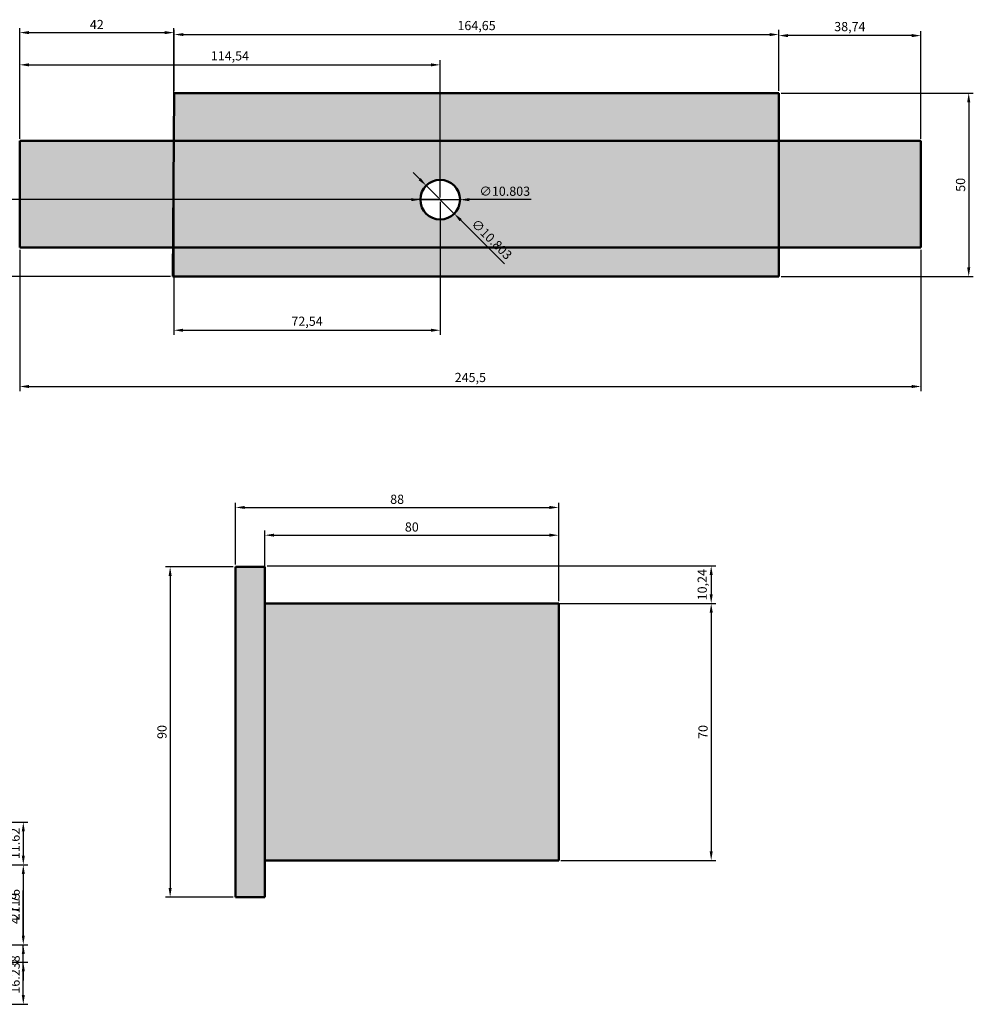
# Model space of a CAD drawing. Units: millimetres. Extents: x 1248 to 2192, y 1962 to 2325.
# Tile 3 of 4: x 1457 to 1717, y 1973 to 2241. Entities that reach past the tile are written whole.
import ezdxf

# ---------------------------------------------------------------- set-up
doc = ezdxf.new("R2010")
doc.units = ezdxf.units.MM
for name, color, linetype, lineweight in [('M-DIMS', 2, 'Continuous', 25), ('M-HATC', 8, 'Continuous', 18), ('M-OUTL', 7, 'Continuous', 50)]:
    doc.layers.add(name, color=color, linetype=linetype, lineweight=lineweight)
doc.styles.get("Standard").update_dxf_attribs({"font": 'arial.ttf'})
doc.dimstyles.new('ISO-25', dxfattribs={"dimtxt": 2.5, "dimasz": 2.5, "dimexe": 1.25, "dimexo": 0.625, "dimtad": 1, "dimtxsty": 'Standard', "dimcen": 2.5, "dimadec": 0, "dimazin": 0, "dimtfac": 1, "dimtmove": 0, "dimatfit": 3, "dimfxl": 1, "dimarcsym": 0})

# ---------------------------------------------------------------- blocks, each defined once
blk = doc.blocks.new('*D12')
at = {"layer": 'Defpoints', "color": 0, "transparency": 16777216}
for p in [(1499.26, 2237.4), (1457.26, 2207.89), (1499.26, 2207.89)]:
    blk.add_point(p, dxfattribs=at)
at = {"layer": 'M-DIMS', "color": 0, "lineweight": -2, "transparency": 16777216}
for p, q in [((1457.26, 2208.51), (1457.26, 2238.65)), ((1459.76, 2237.4), (1496.76, 2237.4)), ((1499.26, 2208.51), (1499.26, 2238.65))]:
    blk.add_line(p, q, dxfattribs=at)
at = {"layer": 'M-DIMS', "color": 0, "transparency": 16777216}
for points in [[(1459.76, 2237.82), (1459.76, 2236.98), (1457.26, 2237.4)], [(1496.76, 2237.82), (1496.76, 2236.98), (1499.26, 2237.4)]]:
    blk.add_solid(points, dxfattribs=at)
at = {"layer": 'M-DIMS', "color": 0, "transparency": 16777216, "insert": (1478.26, 2239.28), "char_height": 2.5, "attachment_point": 5}
blk.add_mtext('42', dxfattribs=at)
blk = doc.blocks.new('*D13')
at = {"layer": 'Defpoints', "color": 0, "transparency": 16777216}
for p in [(1664.02, 2236.87), (1499.37, 2220.93), (1664.02, 2220.93)]:
    blk.add_point(p, dxfattribs=at)
at = {"layer": 'M-DIMS', "color": 0, "lineweight": -2, "transparency": 16777216}
for p, q in [((1499.37, 2221.56), (1499.37, 2238.12)), ((1501.87, 2236.87), (1661.52, 2236.87)), ((1664.02, 2221.56), (1664.02, 2238.12))]:
    blk.add_line(p, q, dxfattribs=at)
at = {"layer": 'M-DIMS', "color": 0, "transparency": 16777216}
for points in [[(1501.87, 2237.28), (1501.87, 2236.45), (1499.37, 2236.87)], [(1661.52, 2237.28), (1661.52, 2236.45), (1664.02, 2236.87)]]:
    blk.add_solid(points, dxfattribs=at)
at = {"layer": 'M-DIMS', "color": 0, "transparency": 16777216, "insert": (1581.7, 2239), "char_height": 2.5, "attachment_point": 5}
blk.add_mtext('164,65', dxfattribs=at)
blk = doc.blocks.new('*D14')
at = {"layer": 'Defpoints', "color": 0, "transparency": 16777216}
for p in [(1664.02, 2236.59), (1664.02, 2220.93), (1702.76, 2207.89)]:
    blk.add_point(p, dxfattribs=at)
at = {"layer": 'M-DIMS', "color": 0, "lineweight": -2, "transparency": 16777216}
for p, q in [((1664.02, 2221.56), (1664.02, 2237.84)), ((1702.76, 2208.51), (1702.76, 2237.84)), ((1700.26, 2236.59), (1666.52, 2236.59))]:
    blk.add_line(p, q, dxfattribs=at)
at = {"layer": 'M-DIMS', "color": 0, "transparency": 16777216}
for points in [[(1666.52, 2237.01), (1666.52, 2236.17), (1664.02, 2236.59)], [(1700.26, 2237.01), (1700.26, 2236.17), (1702.76, 2236.59)]]:
    blk.add_solid(points, dxfattribs=at)
at = {"layer": 'M-DIMS', "color": 0, "transparency": 16777216, "insert": (1683.39, 2238.72), "char_height": 2.5, "attachment_point": 5}
blk.add_mtext('38,74', dxfattribs=at)
blk = doc.blocks.new('*D15')
at = {"layer": 'Defpoints', "color": 0, "transparency": 16777216}
for p in [(1457.26, 2178.86), (1702.76, 2178.86), (1702.76, 2141.01)]:
    blk.add_point(p, dxfattribs=at)
at = {"layer": 'M-DIMS', "color": 0, "lineweight": -2, "transparency": 16777216}
for p, q in [((1457.26, 2178.23), (1457.26, 2139.76)), ((1702.76, 2178.23), (1702.76, 2139.76)), ((1459.76, 2141.01), (1700.26, 2141.01))]:
    blk.add_line(p, q, dxfattribs=at)
at = {"layer": 'M-DIMS', "color": 0, "transparency": 16777216}
for points in [[(1459.76, 2141.43), (1459.76, 2140.59), (1457.26, 2141.01)], [(1700.26, 2141.43), (1700.26, 2140.59), (1702.76, 2141.01)]]:
    blk.add_solid(points, dxfattribs=at)
at = {"layer": 'M-DIMS', "color": 0, "transparency": 16777216, "insert": (1580.01, 2143.14), "char_height": 2.5, "attachment_point": 5}
blk.add_mtext('245,5', dxfattribs=at)
blk = doc.blocks.new('*D16')
at = {"layer": 'Defpoints', "color": 0, "transparency": 16777216}
for p in [(1571.8, 2228.62), (1457.26, 2207.89), (1571.8, 2191.9)]:
    blk.add_point(p, dxfattribs=at)
at = {"layer": 'M-DIMS', "color": 0, "lineweight": -2, "transparency": 16777216}
for p, q in [((1457.26, 2208.51), (1457.26, 2229.87)), ((1571.8, 2192.53), (1571.8, 2229.87)), ((1459.76, 2228.62), (1569.3, 2228.62))]:
    blk.add_line(p, q, dxfattribs=at)
at = {"layer": 'M-DIMS', "color": 0, "transparency": 16777216}
for points in [[(1459.76, 2229.04), (1459.76, 2228.2), (1457.26, 2228.62)], [(1569.3, 2229.04), (1569.3, 2228.2), (1571.8, 2228.62)]]:
    blk.add_solid(points, dxfattribs=at)
at = {"layer": 'M-DIMS', "color": 0, "transparency": 16777216, "insert": (1514.53, 2230.75), "char_height": 2.5, "attachment_point": 5}
blk.add_mtext('114,54', dxfattribs=at)
blk = doc.blocks.new('*D17')
at = {"layer": 'Defpoints', "color": 0, "transparency": 16777216}
for p in [(1499.26, 2207.89), (1571.8, 2191.9), (1571.8, 2156.33)]:
    blk.add_point(p, dxfattribs=at)
at = {"layer": 'M-DIMS', "color": 0, "lineweight": -2, "transparency": 16777216}
for p, q in [((1499.26, 2207.26), (1499.26, 2155.08)), ((1571.8, 2191.28), (1571.8, 2155.08)), ((1501.76, 2156.33), (1569.3, 2156.33))]:
    blk.add_line(p, q, dxfattribs=at)
at = {"layer": 'M-DIMS', "color": 0, "transparency": 16777216}
for points in [[(1501.76, 2156.75), (1501.76, 2155.91), (1499.26, 2156.33)], [(1569.3, 2156.75), (1569.3, 2155.91), (1571.8, 2156.33)]]:
    blk.add_solid(points, dxfattribs=at)
at = {"layer": 'M-DIMS', "color": 0, "transparency": 16777216, "insert": (1535.53, 2158.46), "char_height": 2.5, "attachment_point": 5}
blk.add_mtext('72,54', dxfattribs=at)
blk = doc.blocks.new('*D18')
at = {"layer": 'Defpoints', "color": 0, "transparency": 16777216}
for p in [(1516.07, 2091.9), (1498.24, 2001.9), (1516.07, 2001.9)]:
    blk.add_point(p, dxfattribs=at)
at = {"layer": 'M-DIMS', "color": 0, "lineweight": -2, "transparency": 16777216}
for p, q in [((1515.45, 2091.9), (1496.99, 2091.9)), ((1498.24, 2089.4), (1498.24, 2004.4)), ((1515.45, 2001.9), (1496.99, 2001.9))]:
    blk.add_line(p, q, dxfattribs=at)
at = {"layer": 'M-DIMS', "color": 0, "transparency": 16777216}
for points in [[(1497.82, 2089.4), (1498.66, 2089.4), (1498.24, 2091.9)], [(1497.82, 2004.4), (1498.66, 2004.4), (1498.24, 2001.9)]]:
    blk.add_solid(points, dxfattribs=at)
at = {"layer": 'M-DIMS', "color": 0, "transparency": 16777216, "insert": (1496.34, 2046.9), "char_height": 2.5, "attachment_point": 5, "rotation": 90}
blk.add_mtext('90', dxfattribs=at)
blk = doc.blocks.new('*D19')
at = {"layer": 'Defpoints', "color": 0, "transparency": 16777216}
for p in [(1604.07, 2100.5), (1524.07, 2081.9), (1604.07, 2081.9)]:
    blk.add_point(p, dxfattribs=at)
at = {"layer": 'M-DIMS', "color": 0, "lineweight": -2, "transparency": 16777216}
for p, q in [((1524.07, 2082.53), (1524.07, 2101.75)), ((1526.57, 2100.5), (1601.57, 2100.5)), ((1604.07, 2082.53), (1604.07, 2101.75))]:
    blk.add_line(p, q, dxfattribs=at)
at = {"layer": 'M-DIMS', "color": 0, "transparency": 16777216}
for points in [[(1526.57, 2100.92), (1526.57, 2100.09), (1524.07, 2100.5)], [(1601.57, 2100.92), (1601.57, 2100.09), (1604.07, 2100.5)]]:
    blk.add_solid(points, dxfattribs=at)
at = {"layer": 'M-DIMS', "color": 0, "transparency": 16777216, "insert": (1564.07, 2102.41), "char_height": 2.5, "attachment_point": 5}
blk.add_mtext('80', dxfattribs=at)
blk = doc.blocks.new('*D20')
at = {"layer": 'Defpoints', "color": 0, "transparency": 16777216}
for p in [(1604.07, 2108.06), (1516.07, 2091.9), (1604.07, 2081.9)]:
    blk.add_point(p, dxfattribs=at)
at = {"layer": 'M-DIMS', "color": 0, "lineweight": -2, "transparency": 16777216}
for p, q in [((1516.07, 2092.53), (1516.07, 2109.31)), ((1604.07, 2082.53), (1604.07, 2109.31)), ((1518.57, 2108.06), (1601.57, 2108.06))]:
    blk.add_line(p, q, dxfattribs=at)
at = {"layer": 'M-DIMS', "color": 0, "transparency": 16777216}
for points in [[(1518.57, 2108.47), (1518.57, 2107.64), (1516.07, 2108.06)], [(1601.57, 2108.47), (1601.57, 2107.64), (1604.07, 2108.06)]]:
    blk.add_solid(points, dxfattribs=at)
at = {"layer": 'M-DIMS', "color": 0, "transparency": 16777216, "insert": (1560.07, 2109.96), "char_height": 2.5, "attachment_point": 5}
blk.add_mtext('88', dxfattribs=at)
blk = doc.blocks.new('*D21')
at = {"layer": 'Defpoints', "color": 0, "transparency": 16777216}
for p in [(1604.07, 2081.9), (1604.07, 2011.9), (1645.62, 2011.9)]:
    blk.add_point(p, dxfattribs=at)
at = {"layer": 'M-DIMS', "color": 0, "lineweight": -2, "transparency": 16777216}
for p, q in [((1604.7, 2081.9), (1646.87, 2081.9)), ((1645.62, 2079.4), (1645.62, 2014.4)), ((1604.7, 2011.9), (1646.87, 2011.9))]:
    blk.add_line(p, q, dxfattribs=at)
at = {"layer": 'M-DIMS', "color": 0, "transparency": 16777216}
for points in [[(1645.2, 2079.4), (1646.04, 2079.4), (1645.62, 2081.9)], [(1645.2, 2014.4), (1646.04, 2014.4), (1645.62, 2011.9)]]:
    blk.add_solid(points, dxfattribs=at)
at = {"layer": 'M-DIMS', "color": 0, "transparency": 16777216, "insert": (1643.72, 2046.9), "char_height": 2.5, "attachment_point": 5, "rotation": 90}
blk.add_mtext('70', dxfattribs=at)
blk = doc.blocks.new('*D22')
at = {"layer": 'Defpoints', "color": 0, "transparency": 16777216}
for p in [(1524.07, 2092.14), (1524.07, 2081.9), (1645.62, 2081.9)]:
    blk.add_point(p, dxfattribs=at)
at = {"layer": 'M-DIMS', "color": 0, "lineweight": -2, "transparency": 16777216}
for p, q in [((1524.7, 2092.14), (1646.87, 2092.14)), ((1645.62, 2089.64), (1645.62, 2084.4)), ((1524.7, 2081.9), (1646.87, 2081.9))]:
    blk.add_line(p, q, dxfattribs=at)
at = {"layer": 'M-DIMS', "color": 0, "transparency": 16777216}
for points in [[(1645.2, 2089.64), (1646.04, 2089.64), (1645.62, 2092.14)], [(1645.2, 2084.4), (1646.04, 2084.4), (1645.62, 2081.9)]]:
    blk.add_solid(points, dxfattribs=at)
at = {"layer": 'M-DIMS', "color": 0, "transparency": 16777216, "insert": (1643.49, 2087.02), "char_height": 2.5, "attachment_point": 5, "rotation": 90}
blk.add_mtext('10,24', dxfattribs=at)
blk = doc.blocks.new('*D38')
at = {"layer": 'Defpoints', "color": 0, "transparency": 16777216}
for p in [(1664.02, 2220.93), (1664.02, 2170.93), (1715.76, 2170.93)]:
    blk.add_point(p, dxfattribs=at)
at = {"layer": 'M-DIMS', "color": 0, "lineweight": -2, "transparency": 16777216}
for p, q in [((1664.65, 2220.93), (1717.01, 2220.93)), ((1715.76, 2218.43), (1715.76, 2173.43)), ((1664.65, 2170.93), (1717.01, 2170.93))]:
    blk.add_line(p, q, dxfattribs=at)
at = {"layer": 'M-DIMS', "color": 0, "transparency": 16777216}
for points in [[(1715.34, 2218.43), (1716.18, 2218.43), (1715.76, 2220.93)], [(1715.34, 2173.43), (1716.18, 2173.43), (1715.76, 2170.93)]]:
    blk.add_solid(points, dxfattribs=at)
at = {"layer": 'M-DIMS', "color": 0, "transparency": 16777216, "insert": (1713.86, 2195.93), "char_height": 2.5, "attachment_point": 5, "rotation": 90}
blk.add_mtext('50', dxfattribs=at)
blk = doc.blocks.new('*D40')
at = {"layer": 'Defpoints', "color": 0, "transparency": 16777216}
for p in [(1571.8, 2191.9), (1444.26, 2170.93), (1498.95, 2170.93)]:
    blk.add_point(p, dxfattribs=at)
at = {"layer": 'M-DIMS', "color": 0, "lineweight": -2, "transparency": 16777216}
for p, q in [((1571.17, 2191.9), (1443.01, 2191.9)), ((1444.26, 2189.4), (1444.26, 2173.43)), ((1498.32, 2170.93), (1443.01, 2170.93))]:
    blk.add_line(p, q, dxfattribs=at)
at = {"layer": 'M-DIMS', "color": 0, "transparency": 16777216}
for points in [[(1443.84, 2189.4), (1444.68, 2189.4), (1444.26, 2191.9)], [(1443.84, 2173.43), (1444.68, 2173.43), (1444.26, 2170.93)]]:
    blk.add_solid(points, dxfattribs=at)
at = {"layer": 'M-DIMS', "color": 0, "transparency": 16777216, "insert": (1442.36, 2181.42), "char_height": 2.5, "attachment_point": 5, "rotation": 90}
blk.add_mtext('20.97', dxfattribs=at)
blk = doc.blocks.new('*D43')
at = {"layer": 'Defpoints', "color": 0, "transparency": 16777216}
for p in [(1448.89, 2010.72), (1448.64, 1988.96), (1458.24, 1988.96)]:
    blk.add_point(p, dxfattribs=at)
at = {"layer": 'M-DIMS', "color": 0, "lineweight": -2, "transparency": 16777216}
for p, q in [((1449.52, 2010.72), (1459.49, 2010.72)), ((1458.24, 2008.22), (1458.24, 1991.46)), ((1449.26, 1988.96), (1459.49, 1988.96))]:
    blk.add_line(p, q, dxfattribs=at)
at = {"layer": 'M-DIMS', "color": 0, "transparency": 16777216}
for points in [[(1457.83, 2008.22), (1458.66, 2008.22), (1458.24, 2010.72)], [(1457.83, 1991.46), (1458.66, 1991.46), (1458.24, 1988.96)]]:
    blk.add_solid(points, dxfattribs=at)
at = {"layer": 'M-DIMS', "color": 0, "transparency": 16777216, "insert": (1456.34, 1999.84), "char_height": 2.5, "attachment_point": 5, "rotation": 90}
blk.add_mtext('21.76', dxfattribs=at)
blk = doc.blocks.new('*D44')
at = {"layer": 'Defpoints', "color": 0, "transparency": 16777216}
for p in [(1429.82, 2022.34), (1448.89, 2010.72), (1458.24, 2010.72)]:
    blk.add_point(p, dxfattribs=at)
at = {"layer": 'M-DIMS', "color": 0, "lineweight": -2, "transparency": 16777216}
for p, q in [((1430.45, 2022.34), (1459.49, 2022.34)), ((1458.24, 2019.84), (1458.24, 2013.22)), ((1449.52, 2010.72), (1459.49, 2010.72))]:
    blk.add_line(p, q, dxfattribs=at)
at = {"layer": 'M-DIMS', "color": 0, "transparency": 16777216}
for points in [[(1457.83, 2019.84), (1458.66, 2019.84), (1458.24, 2022.34)], [(1457.83, 2013.22), (1458.66, 2013.22), (1458.24, 2010.72)]]:
    blk.add_solid(points, dxfattribs=at)
at = {"layer": 'M-DIMS', "color": 0, "transparency": 16777216, "insert": (1456.34, 2016.53), "char_height": 2.5, "attachment_point": 5, "rotation": 90}
blk.add_mtext('11.62', dxfattribs=at)
blk = doc.blocks.new('*D45')
at = {"layer": 'Defpoints', "color": 0, "transparency": 16777216}
for p in [(1448.64, 1988.96), (1458.24, 1988.96), (1437.87, 1972.72)]:
    blk.add_point(p, dxfattribs=at)
at = {"layer": 'M-DIMS', "color": 0, "lineweight": -2, "transparency": 16777216}
for p, q in [((1449.26, 1988.96), (1459.49, 1988.96)), ((1458.24, 1975.22), (1458.24, 1986.46)), ((1438.49, 1972.72), (1459.49, 1972.72))]:
    blk.add_line(p, q, dxfattribs=at)
at = {"layer": 'M-DIMS', "color": 0, "transparency": 16777216}
for points in [[(1457.83, 1986.46), (1458.66, 1986.46), (1458.24, 1988.96)], [(1457.83, 1975.22), (1458.66, 1975.22), (1458.24, 1972.72)]]:
    blk.add_solid(points, dxfattribs=at)
at = {"layer": 'M-DIMS', "color": 0, "transparency": 16777216, "insert": (1456.34, 1980.84), "char_height": 2.5, "attachment_point": 5, "rotation": 90}
blk.add_mtext('16.238', dxfattribs=at)
blk = doc.blocks.new('*D49')
at = {"layer": 'Defpoints', "color": 0, "transparency": 16777216}
for p in [(1428.64, 1988.96), (1458.24, 1988.96), (1422.43, 1984.24)]:
    blk.add_point(p, dxfattribs=at)
at = {"layer": 'M-DIMS', "color": 0, "lineweight": -2, "transparency": 16777216}
for p, q in [((1458.24, 1991.46), (1458.24, 2003.75)), ((1429.26, 1988.96), (1459.49, 1988.96)), ((1458.24, 1984.24), (1458.24, 1988.96)), ((1423.06, 1984.24), (1459.49, 1984.24)), ((1458.24, 1981.74), (1458.24, 1979.24))]:
    blk.add_line(p, q, dxfattribs=at)
at = {"layer": 'M-DIMS', "color": 0, "transparency": 16777216}
for points in [[(1457.83, 1991.46), (1458.66, 1991.46), (1458.24, 1988.96)], [(1457.83, 1981.74), (1458.66, 1981.74), (1458.24, 1984.24)]]:
    blk.add_solid(points, dxfattribs=at)
at = {"layer": 'M-DIMS', "color": 0, "transparency": 16777216, "insert": (1456.34, 1998.85), "char_height": 2.5, "attachment_point": 5, "rotation": 90}
blk.add_mtext('4.719', dxfattribs=at)
blk = doc.blocks.new('*D60')
at = {"layer": 'Defpoints', "color": 0, "transparency": 16777216}
for p in [(1566.4, 2191.9), (1577.2, 2191.9)]:
    blk.add_point(p, dxfattribs=at)
at = {"layer": 'M-DIMS', "color": 0, "lineweight": -2, "transparency": 16777216}
for p, q in [((1563.9, 2191.9), (1561.4, 2191.9)), ((1566.4, 2191.9), (1577.2, 2191.9)), ((1596.55, 2191.9), (1579.7, 2191.9))]:
    blk.add_line(p, q, dxfattribs=at)
at = {"layer": 'M-DIMS', "color": 0, "transparency": 16777216}
for points in [[(1563.9, 2192.32), (1563.9, 2191.49), (1566.4, 2191.9)], [(1579.7, 2192.32), (1579.7, 2191.48), (1577.2, 2191.9)]]:
    blk.add_solid(points, dxfattribs=at)
at = {"layer": 'M-DIMS', "color": 0, "transparency": 16777216, "insert": (1589.38, 2193.87), "char_height": 2.5, "attachment_point": 5, "rotation": 359.9906}
blk.add_mtext('∅10.803', dxfattribs=at)
blk = doc.blocks.new('*D77')
at = {"layer": 'Defpoints', "color": 0, "transparency": 16777216}
for p in [(1567.98, 2195.72), (1575.62, 2188.08)]:
    blk.add_point(p, dxfattribs=at)
at = {"layer": 'M-DIMS', "color": 0, "lineweight": -2, "transparency": 16777216}
for p, q in [((1566.21, 2197.49), (1564.45, 2199.26)), ((1567.98, 2195.72), (1575.62, 2188.08)), ((1589.3, 2174.4), (1577.39, 2186.31))]:
    blk.add_line(p, q, dxfattribs=at)
at = {"layer": 'M-DIMS', "color": 0, "transparency": 16777216}
for points in [[(1566.51, 2197.78), (1565.92, 2197.19), (1567.98, 2195.72)], [(1577.68, 2186.61), (1577.09, 2186.02), (1575.62, 2188.08)]]:
    blk.add_solid(points, dxfattribs=at)
at = {"layer": 'M-DIMS', "color": 0, "transparency": 16777216, "insert": (1585.62, 2180.87), "char_height": 2.5, "attachment_point": 5, "rotation": 314.9948}
blk.add_mtext('∅10.803', dxfattribs=at)

msp = doc.modelspace()

# ---------------------------------------------------------------- hatches: boundary and pattern name
at = {"layer": 'M-HATC'}
h = msp.add_hatch(color=256, dxfattribs=at)
h.set_gradient(color1=(114, 116, 48), color2=(114, 116, 48))
h.paths.add_polyline_path([(1499.2611, 2207.8886), (1457.2612, 2207.8886), (1457.2612, 2178.8583), (1499.0166, 2178.8583)])
h.paths.add_polyline_path([(1664.0202, 2207.8886), (1499.2611, 2207.8886), (1499.0166, 2178.8583), (1619.3839, 2178.8583), (1664.0202, 2178.8583)])
h.paths.add_polyline_path([(1577.2015, 2191.9009, -1), (1566.3981, 2191.9009, -1)], flags=16)
h.paths.add_polyline_path([(1702.7612, 2207.8886), (1664.0202, 2207.8886), (1664.0202, 2178.8583), (1702.7612, 2178.8583)])
h.paths.add_polyline_path([(1664.0202, 2220.9312), (1499.371, 2220.9312), (1499.2611, 2207.8886), (1664.0202, 2207.8886)])
h.paths.add_polyline_path([(1664.0202, 2178.8583), (1619.3839, 2178.8583), (1499.0166, 2178.8583), (1498.9499, 2170.9312), (1664.0202, 2170.9312)])
h = msp.add_hatch(color=256, dxfattribs=at)
h.set_gradient(color1=(19, 103, 52), color2=(19, 103, 52))
h.paths.add_polyline_path([(1524.0714, 2011.9002), (1604.0714, 2011.9002), (1604.0714, 2081.9002), (1524.0714, 2081.9002)])
h.paths.add_polyline_path([(1516.0714, 2001.9002), (1524.0714, 2001.9002), (1524.0714, 2091.9002), (1516.0714, 2091.9002)])

# ---------------------------------------------------------------- linework, layer by layer
at = {"layer": 'M-OUTL'}
for p, q in [((1498.9499, 2170.9312), (1499.371, 2220.9312)), ((1499.371, 2220.9312), (1664.0202, 2220.9312)), ((1664.0202, 2220.9312), (1664.0202, 2170.9312)), ((1499.2611, 2207.8886), (1457.2612, 2207.8886)), ((1457.2612, 2207.8886), (1457.2612, 2178.8583)), ((1499.2611, 2207.8886), (1702.7612, 2207.8886)), ((1702.7612, 2207.8886), (1702.7612, 2178.8583)), ((1619.3839, 2178.8583), (1457.2612, 2178.8583)), ((1702.7612, 2178.8583), (1619.3839, 2178.8583)), ((1664.0202, 2170.9312), (1498.9499, 2170.9312)), ((1516.0714, 2091.9002), (1516.0714, 2001.9002)), ((1524.0714, 2091.9002), (1516.0714, 2091.9002)), ((1524.0714, 2001.9002), (1524.0714, 2091.9002)), ((1524.0714, 2091.9002), (1524.0714, 2081.9002)), ((1524.0714, 2081.9002), (1604.0714, 2081.9002)), ((1604.0714, 2081.9002), (1604.0714, 2011.9002)), ((1604.0714, 2011.9002), (1524.0714, 2011.9002)), ((1516.0714, 2001.9002), (1524.0714, 2001.9002))]:
    msp.add_line(p, q, dxfattribs=at)
msp.add_circle((1571.7998, 2191.9009), 5.4017, dxfattribs=at)

# ---------------------------------------------------------------- dimensions: what is measured, and where the dimension line sits
at = {"layer": 'M-DIMS'}
for base, p1, p2, picture, middle in [((1499.2611, 2237.3998), (1457.2612, 2207.8886), (1499.2611, 2207.8886), '*D12', (1478.2612, 2239.2799)), ((1664.0202, 2236.868), (1499.371, 2220.9312), (1664.0202, 2220.9312), '*D13', (1581.6956, 2238.9954)), ((1664.0202, 2236.5911), (1702.7612, 2207.8886), (1664.0202, 2220.9312), '*D14', (1683.3907, 2238.7185)), ((1571.7998, 2228.6185), (1457.2612, 2207.8886), (1571.7998, 2191.9009), '*D16', (1514.5305, 2230.7459)), ((1571.7998, 2156.3293), (1499.2611, 2207.8886), (1571.7998, 2191.9009), '*D17', (1535.5305, 2158.4567)), ((1702.7612, 2141.0116), (1457.2612, 2178.8583), (1702.7612, 2178.8583), '*D15', (1580.0112, 2143.1389)), ((1604.0714, 2108.0561), (1516.0714, 2091.9002), (1604.0714, 2081.9002), '*D20', (1560.0714, 2109.9575)), ((1604.0714, 2100.5047), (1524.0714, 2081.9002), (1604.0714, 2081.9002), '*D19', (1564.0714, 2102.4061))]:
    dim = msp.add_linear_dim(base=base, p1=p1, p2=p2, dimstyle='ISO-25', override={"dimclrd": 0, "dimclre": 0, "dimclrt": 0}, dxfattribs=at)
    dim.commit()
    dim.dimension.update_dxf_attribs({"geometry": picture, "text_midpoint": middle})
for base, p1, p2, override, picture, middle in [((1715.7612, 2170.9312), (1664.0202, 2220.9312), (1664.0202, 2170.9312), {"dimdec": 0, "dimlfac": 1, "dimrnd": 0, "dimzin": 0, "dimdsep": 46, "dimlunit": 2}, '*D38', (1713.8598, 2195.9312)), ((1444.2612, 2170.9312), (1571.7998, 2191.9009), (1498.9499, 2170.9312), {"dimdec": 2, "dimlfac": 1, "dimrnd": 0, "dimzin": 0, "dimdsep": 46, "dimlunit": 2}, '*D40', (1442.3598, 2181.4161)), ((1645.6199, 2081.9002), (1524.0714, 2092.1399), (1524.0714, 2081.9002), {"dimclrd": 0, "dimclre": 0, "dimclrt": 0}, '*D22', (1643.4925, 2087.02)), ((1498.2389, 2001.9002), (1516.0714, 2091.9002), (1516.0714, 2001.9002), {"dimclrd": 0, "dimclre": 0, "dimclrt": 0}, '*D18', (1496.3375, 2046.9002)), ((1645.6199, 2011.9002), (1604.0714, 2081.9002), (1604.0714, 2011.9002), {"dimclrd": 0, "dimclre": 0, "dimclrt": 0}, '*D21', (1643.7185, 2046.9002)), ((1458.2445, 2010.7199), (1429.824, 2022.341), (1448.8945, 2010.7199), {"dimdec": 2, "dimlfac": 1, "dimrnd": 0, "dimzin": 0, "dimdsep": 46, "dimlunit": 2}, '*D44', (1456.3431, 2016.5305)), ((1458.2445, 1988.958), (1448.8945, 2010.7199), (1448.6368, 1988.958), {"dimdec": 2, "dimlfac": 1, "dimrnd": 0, "dimzin": 0, "dimdsep": 46, "dimlunit": 2}, '*D43', (1456.3431, 1999.8389)), ((1458.2445, 1988.958), (1422.4308, 1984.2387), (1428.6368, 1988.958), {"dimdec": 3, "dimlfac": 1, "dimrnd": 0, "dimzin": 0, "dimdsep": 46, "dimlunit": 2}, '*D49', (1456.3431, 1998.854)), ((1458.2445, 1988.958), (1437.8682, 1972.7199), (1448.6368, 1988.958), {"dimdec": 3, "dimlfac": 1, "dimrnd": 0, "dimzin": 0, "dimdsep": 46, "dimlunit": 2}, '*D45', (1456.3422, 1980.8389))]:
    dim = msp.add_linear_dim(base=base, p1=p1, p2=p2, angle=90, dimstyle='ISO-25', override=override, dxfattribs=at)
    dim.commit()
    dim.dimension.update_dxf_attribs({"geometry": picture, "text_midpoint": middle})
for p1, p2, picture, middle in [((1567.9806, 2195.7208), (1575.619, 2188.081), '*D77', (1584.2268, 2179.4717)), ((1566.3981, 2191.9018), (1577.2015, 2191.9), '*D60', (1589.3758, 2191.898))]:
    dim = msp.add_diameter_dim_2p(p1=p1, p2=p2, dimstyle='ISO-25', override={"dimdec": 3, "dimlfac": 1, "dimrnd": 0, "dimzin": 0, "dimdsep": 46, "dimlunit": 2}, dxfattribs=at)
    dim.commit()
    dim.dimension.update_dxf_attribs({"geometry": picture, "text_midpoint": middle, "dimtype": 163})

doc.saveas('drawing.dxf')
